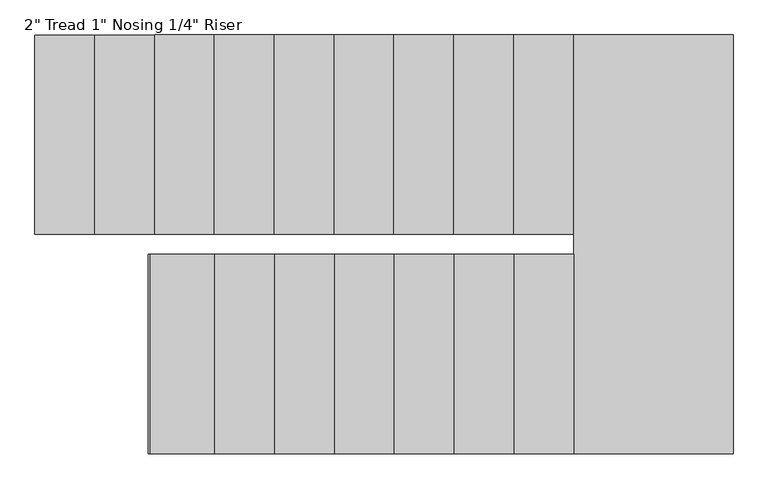
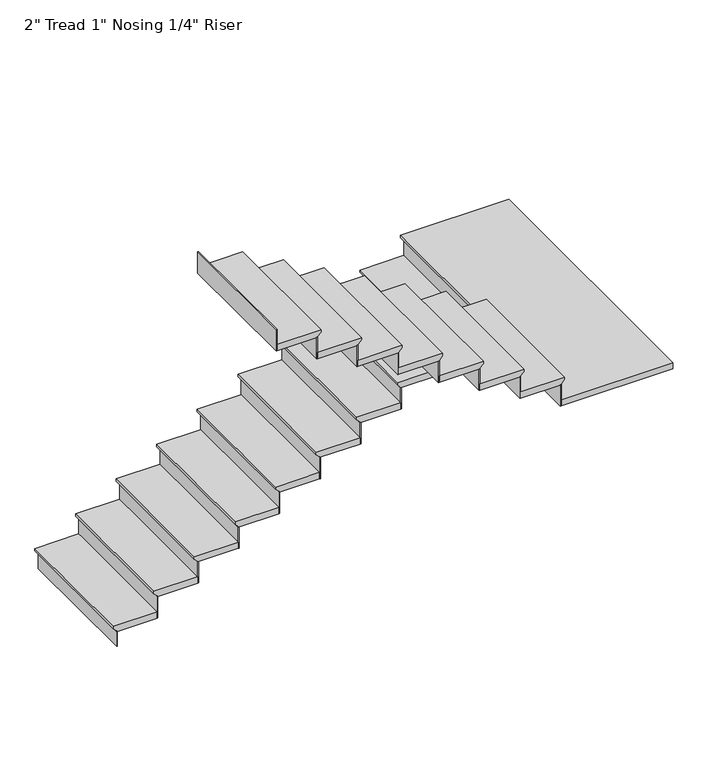
"""IFC4 building model written with IfcOpenShell, lengths in millimetres: stair flight geometry."""

from ifc_helpers import new_model, si_unit, origin, place, context, project, spatial, faceted_brep, source, transform, mapped, element, save


def stair_flight_7f10be43(model_context):
    return source(origin(), model_context, "Body", "Brep", [
        faceted_brep([(-12755.7436606, -2894.3024127, 3503.0833333), (-12755.7436606, -2894.3024127, 3522.1333333), (-12755.7436606, -1878.3024127, 3522.1333333), (-12755.7436606, -1878.3024127, 3503.0833333), (-12730.3436606, -2894.3024127, 3477.6833333), (-12730.3436606, -1878.3024127, 3477.6833333), (-12425.5436606, -2894.3024127, 3522.1333333), (-12425.5436606, -1878.3024127, 3522.1333333), (-12730.3436606, -1878.3024127, 3471.3333333), (-12425.5436606, -1878.3024127, 3471.3333333), (-12425.5436606, -2894.3024127, 3471.3333333), (-12730.3436606, -2894.3024127, 3471.3333333)], [[[0, 1, 2, 3]], [[4, 0, 3, 5]], [[2, 1, 6, 7]], [[8, 9, 10, 11]], [[2, 7, 9, 8, 5, 3]], [[8, 11, 4, 5]], [[6, 1, 0, 4, 11, 10]], [[7, 6, 10, 9]]]),
        faceted_brep([(-12730.3436606, -2894.3024127, 3471.3333333), (-12730.3436606, -2894.3024127, 3352.8), (-12723.9936606, -2894.3024127, 3352.8), (-12723.9936606, -2894.3024127, 3471.3333333), (-12730.3436606, -1878.3024127, 3471.3333333), (-12723.9936606, -1878.3024127, 3471.3333333), (-12723.9936606, -1878.3024127, 3352.8), (-12730.3436606, -1878.3024127, 3352.8)], [[[0, 1, 2, 3]], [[4, 5, 6, 7]], [[1, 0, 4, 7]], [[2, 1, 7, 6]], [[3, 2, 6, 5]], [[0, 3, 5, 4]]]),
        faceted_brep([(-12425.5436606, -2894.3024127, 3640.6666667), (-12425.5436606, -2894.3024127, 3471.3333333), (-12419.1936606, -2894.3024127, 3471.3333333), (-12419.1936606, -2894.3024127, 3640.6666667), (-12425.5436606, -1878.3024127, 3640.6666667), (-12419.1936606, -1878.3024127, 3640.6666667), (-12419.1936606, -1878.3024127, 3471.3333333), (-12425.5436606, -1878.3024127, 3471.3333333)], [[[0, 1, 2, 3]], [[4, 5, 6, 7]], [[1, 0, 4, 7]], [[2, 1, 7, 6]], [[3, 2, 6, 5]], [[0, 3, 5, 4]]]),
        faceted_brep([(-12450.9436606, -1878.3024127, 3691.4666667), (-12450.9436606, -2894.3024127, 3691.4666667), (-12120.7436606, -2894.3024127, 3691.4666667), (-12120.7436606, -1878.3024127, 3691.4666667), (-12425.5436606, -1878.3024127, 3640.6666667), (-12120.7436606, -1878.3024127, 3640.6666667), (-12120.7436606, -2894.3024127, 3640.6666667), (-12425.5436606, -2894.3024127, 3640.6666667), (-12425.5436606, -1878.3024127, 3647.0166667), (-12450.9436606, -1878.3024127, 3672.4166667), (-12425.5436606, -2894.3024127, 3647.0166667), (-12450.9436606, -2894.3024127, 3672.4166667)], [[[0, 1, 2, 3]], [[4, 5, 6, 7]], [[0, 3, 5, 4, 8, 9]], [[4, 7, 10, 8]], [[2, 1, 11, 10, 7, 6]], [[3, 2, 6, 5]], [[11, 1, 0, 9]], [[10, 11, 9, 8]]]),
        faceted_brep([(-12120.7436606, -2894.3024127, 3810.0), (-12120.7436606, -2894.3024127, 3640.6666667), (-12114.3936606, -2894.3024127, 3640.6666667), (-12114.3936606, -2894.3024127, 3810.0), (-12120.7436606, -1878.3024127, 3810.0), (-12114.3936606, -1878.3024127, 3810.0), (-12114.3936606, -1878.3024127, 3640.6666667), (-12120.7436606, -1878.3024127, 3640.6666667)], [[[0, 1, 2, 3]], [[4, 5, 6, 7]], [[1, 0, 4, 7]], [[2, 1, 7, 6]], [[3, 2, 6, 5]], [[0, 3, 5, 4]]]),
        faceted_brep([(-12146.1436606, -1878.3024127, 3860.8), (-12146.1436606, -2894.3024127, 3860.8), (-11815.9436606, -2894.3024127, 3860.8), (-11815.9436606, -1878.3024127, 3860.8), (-12120.7436606, -1878.3024127, 3810.0), (-11815.9436606, -1878.3024127, 3810.0), (-11815.9436606, -2894.3024127, 3810.0), (-12120.7436606, -2894.3024127, 3810.0), (-12120.7436606, -1878.3024127, 3816.35), (-12146.1436606, -1878.3024127, 3841.75), (-12120.7436606, -2894.3024127, 3816.35), (-12146.1436606, -2894.3024127, 3841.75)], [[[0, 1, 2, 3]], [[4, 5, 6, 7]], [[0, 3, 5, 4, 8, 9]], [[4, 7, 10, 8]], [[2, 1, 11, 10, 7, 6]], [[3, 2, 6, 5]], [[11, 1, 0, 9]], [[10, 11, 9, 8]]]),
        faceted_brep([(-11815.9436606, -2894.3024127, 3979.3333333), (-11815.9436606, -2894.3024127, 3810.0), (-11809.5936606, -2894.3024127, 3810.0), (-11809.5936606, -2894.3024127, 3979.3333333), (-11815.9436606, -1878.3024127, 3979.3333333), (-11809.5936606, -1878.3024127, 3979.3333333), (-11809.5936606, -1878.3024127, 3810.0), (-11815.9436606, -1878.3024127, 3810.0)], [[[0, 1, 2, 3]], [[4, 5, 6, 7]], [[1, 0, 4, 7]], [[2, 1, 7, 6]], [[3, 2, 6, 5]], [[0, 3, 5, 4]]]),
        faceted_brep([(-11841.3436606, -1878.3024127, 4030.1333333), (-11841.3436606, -2894.3024127, 4030.1333333), (-11511.1436606, -2894.3024127, 4030.1333333), (-11511.1436606, -1878.3024127, 4030.1333333), (-11815.9436606, -1878.3024127, 3979.3333333), (-11511.1436606, -1878.3024127, 3979.3333333), (-11511.1436606, -2894.3024127, 3979.3333333), (-11815.9436606, -2894.3024127, 3979.3333333), (-11815.9436606, -1878.3024127, 3985.6833333), (-11841.3436606, -1878.3024127, 4011.0833333), (-11815.9436606, -2894.3024127, 3985.6833333), (-11841.3436606, -2894.3024127, 4011.0833333)], [[[0, 1, 2, 3]], [[4, 5, 6, 7]], [[0, 3, 5, 4, 8, 9]], [[4, 7, 10, 8]], [[2, 1, 11, 10, 7, 6]], [[3, 2, 6, 5]], [[11, 1, 0, 9]], [[10, 11, 9, 8]]]),
        faceted_brep([(-11511.1436606, -2894.3024127, 4148.6666667), (-11511.1436606, -2894.3024127, 3979.3333333), (-11504.7936606, -2894.3024127, 3979.3333333), (-11504.7936606, -2894.3024127, 4148.6666667), (-11511.1436606, -1878.3024127, 4148.6666667), (-11504.7936606, -1878.3024127, 4148.6666667), (-11504.7936606, -1878.3024127, 3979.3333333), (-11511.1436606, -1878.3024127, 3979.3333333)], [[[0, 1, 2, 3]], [[4, 5, 6, 7]], [[1, 0, 4, 7]], [[2, 1, 7, 6]], [[3, 2, 6, 5]], [[0, 3, 5, 4]]]),
        faceted_brep([(-11536.5436606, -1878.3024127, 4199.4666667), (-11536.5436606, -2894.3024127, 4199.4666667), (-11206.3436606, -2894.3024127, 4199.4666667), (-11206.3436606, -1878.3024127, 4199.4666667), (-11511.1436606, -1878.3024127, 4148.6666667), (-11206.3436606, -1878.3024127, 4148.6666667), (-11206.3436606, -2894.3024127, 4148.6666667), (-11511.1436606, -2894.3024127, 4148.6666667), (-11511.1436606, -1878.3024127, 4155.0166667), (-11536.5436606, -1878.3024127, 4180.4166667), (-11511.1436606, -2894.3024127, 4155.0166667), (-11536.5436606, -2894.3024127, 4180.4166667)], [[[0, 1, 2, 3]], [[4, 5, 6, 7]], [[0, 3, 5, 4, 8, 9]], [[4, 7, 10, 8]], [[2, 1, 11, 10, 7, 6]], [[3, 2, 6, 5]], [[11, 1, 0, 9]], [[10, 11, 9, 8]]]),
        faceted_brep([(-11206.3436606, -2894.3024127, 4318.0), (-11206.3436606, -2894.3024127, 4148.6666667), (-11199.9936606, -2894.3024127, 4148.6666667), (-11199.9936606, -2894.3024127, 4318.0), (-11206.3436606, -1878.3024127, 4318.0), (-11199.9936606, -1878.3024127, 4318.0), (-11199.9936606, -1878.3024127, 4148.6666667), (-11206.3436606, -1878.3024127, 4148.6666667)], [[[0, 1, 2, 3]], [[4, 5, 6, 7]], [[1, 0, 4, 7]], [[2, 1, 7, 6]], [[3, 2, 6, 5]], [[0, 3, 5, 4]]]),
        faceted_brep([(-11231.7436606, -1878.3024127, 4368.8), (-11231.7436606, -2894.3024127, 4368.8), (-10901.5436606, -2894.3024127, 4368.8), (-10901.5436606, -1878.3024127, 4368.8), (-11206.3436606, -1878.3024127, 4318.0), (-10901.5436606, -1878.3024127, 4318.0), (-10901.5436606, -2894.3024127, 4318.0), (-11206.3436606, -2894.3024127, 4318.0), (-11206.3436606, -1878.3024127, 4324.35), (-11231.7436606, -1878.3024127, 4349.75), (-11206.3436606, -2894.3024127, 4324.35), (-11231.7436606, -2894.3024127, 4349.75)], [[[0, 1, 2, 3]], [[4, 5, 6, 7]], [[0, 3, 5, 4, 8, 9]], [[4, 7, 10, 8]], [[2, 1, 11, 10, 7, 6]], [[3, 2, 6, 5]], [[11, 1, 0, 9]], [[10, 11, 9, 8]]]),
        faceted_brep([(-10901.5436606, -2894.3024127, 4487.3333333), (-10901.5436606, -2894.3024127, 4318.0), (-10895.1936606, -2894.3024127, 4318.0), (-10895.1936606, -2894.3024127, 4487.3333333), (-10901.5436606, -1878.3024127, 4487.3333333), (-10895.1936606, -1878.3024127, 4487.3333333), (-10895.1936606, -1878.3024127, 4318.0), (-10901.5436606, -1878.3024127, 4318.0)], [[[0, 1, 2, 3]], [[4, 5, 6, 7]], [[1, 0, 4, 7]], [[2, 1, 7, 6]], [[3, 2, 6, 5]], [[0, 3, 5, 4]]]),
        faceted_brep([(-10926.9436606, -1878.3024127, 4538.1333333), (-10926.9436606, -2894.3024127, 4538.1333333), (-10596.7436606, -2894.3024127, 4538.1333333), (-10596.7436606, -1878.3024127, 4538.1333333), (-10901.5436606, -1878.3024127, 4487.3333333), (-10596.7436606, -1878.3024127, 4487.3333333), (-10596.7436606, -2894.3024127, 4487.3333333), (-10901.5436606, -2894.3024127, 4487.3333333), (-10901.5436606, -1878.3024127, 4493.6833333), (-10926.9436606, -1878.3024127, 4519.0833333), (-10901.5436606, -2894.3024127, 4493.6833333), (-10926.9436606, -2894.3024127, 4519.0833333)], [[[0, 1, 2, 3]], [[4, 5, 6, 7]], [[0, 3, 5, 4, 8, 9]], [[4, 7, 10, 8]], [[2, 1, 11, 10, 7, 6]], [[3, 2, 6, 5]], [[11, 1, 0, 9]], [[10, 11, 9, 8]]]),
        faceted_brep([(-10596.7436606, -2894.3024127, 4656.6666667), (-10596.7436606, -2894.3024127, 4487.3333333), (-10590.3936606, -2894.3024127, 4487.3333333), (-10590.3936606, -2894.3024127, 4656.6666667), (-10596.7436606, -1878.3024127, 4656.6666667), (-10590.3936606, -1878.3024127, 4656.6666667), (-10590.3936606, -1878.3024127, 4487.3333333), (-10596.7436606, -1878.3024127, 4487.3333333)], [[[0, 1, 2, 3]], [[4, 5, 6, 7]], [[1, 0, 4, 7]], [[2, 1, 7, 6]], [[3, 2, 6, 5]], [[0, 3, 5, 4]]]),
        faceted_brep([(-10622.1436606, -1878.3024127, 4707.4666667), (-10622.1436606, -2894.3024127, 4707.4666667), (-10291.9436606, -2894.3024127, 4707.4666667), (-10291.9436606, -1878.3024127, 4707.4666667), (-10596.7436606, -1878.3024127, 4656.6666667), (-10291.9436606, -1878.3024127, 4656.6666667), (-10291.9436606, -2894.3024127, 4656.6666667), (-10596.7436606, -2894.3024127, 4656.6666667), (-10596.7436606, -1878.3024127, 4663.0166667), (-10622.1436606, -1878.3024127, 4688.4166667), (-10596.7436606, -2894.3024127, 4663.0166667), (-10622.1436606, -2894.3024127, 4688.4166667)], [[[0, 1, 2, 3]], [[4, 5, 6, 7]], [[0, 3, 5, 4, 8, 9]], [[4, 7, 10, 8]], [[2, 1, 11, 10, 7, 6]], [[3, 2, 6, 5]], [[11, 1, 0, 9]], [[10, 11, 9, 8]]]),
        faceted_brep([(-10291.9436606, -2894.3024127, 4826.0), (-10291.9436606, -2894.3024127, 4656.6666667), (-10285.5936606, -2894.3024127, 4656.6666667), (-10285.5936606, -2894.3024127, 4826.0), (-10291.9436606, -1878.3024127, 4826.0), (-10285.5936606, -1878.3024127, 4826.0), (-10285.5936606, -1878.3024127, 4656.6666667), (-10291.9436606, -1878.3024127, 4656.6666667)], [[[0, 1, 2, 3]], [[4, 5, 6, 7]], [[1, 0, 4, 7]], [[2, 1, 7, 6]], [[3, 2, 6, 5]], [[0, 3, 5, 4]]]),
        faceted_brep([(-10317.3436606, -1878.3024127, 4876.8), (-10317.3436606, -2894.3024127, 4876.8), (-9987.1436606, -2894.3024127, 4876.8), (-9987.1436606, -1878.3024127, 4876.8), (-10291.9436606, -1878.3024127, 4826.0), (-9987.1436606, -1878.3024127, 4826.0), (-9987.1436606, -2894.3024127, 4826.0), (-10291.9436606, -2894.3024127, 4826.0), (-10291.9436606, -1878.3024127, 4832.35), (-10317.3436606, -1878.3024127, 4857.75), (-10291.9436606, -2894.3024127, 4832.35), (-10317.3436606, -2894.3024127, 4857.75)], [[[0, 1, 2, 3]], [[4, 5, 6, 7]], [[0, 3, 5, 4, 8, 9]], [[4, 7, 10, 8]], [[2, 1, 11, 10, 7, 6]], [[3, 2, 6, 5]], [[11, 1, 0, 9]], [[10, 11, 9, 8]]]),
        faceted_brep([(-9987.1436606, -2894.3024127, 4995.3333333), (-9987.1436606, -2894.3024127, 4826.0), (-9980.7936606, -2894.3024127, 4826.0), (-9980.7936606, -2894.3024127, 4995.3333333), (-9987.1436606, -1878.3024127, 4995.3333333), (-9980.7936606, -1878.3024127, 4995.3333333), (-9980.7936606, -1878.3024127, 4826.0), (-9987.1436606, -1878.3024127, 4826.0)], [[[0, 1, 2, 3]], [[4, 5, 6, 7]], [[1, 0, 4, 7]], [[2, 1, 7, 6]], [[3, 2, 6, 5]], [[0, 3, 5, 4]]]),
        faceted_brep([(-10037.9436606, -4011.9024127, 5046.1333333), (-9199.7436606, -4011.9024127, 5046.1333333), (-9199.7436606, -1878.3024127, 5046.1333333), (-10012.5436606, -1878.3024127, 5046.1333333), (-10012.5436606, -2995.9024127, 5046.1333333), (-10037.9436606, -2995.9024127, 5046.1333333), (-9199.7436606, -4011.9024127, 4995.3333333), (-10037.9436606, -4011.9024127, 4995.3333333), (-10037.9436606, -2995.9024127, 4995.3333333), (-10012.5436606, -2995.9024127, 4995.3333333), (-10012.5436606, -2894.3024127, 4995.3333333), (-9987.1436606, -2894.3024127, 4995.3333333), (-9987.1436606, -1878.3024127, 4995.3333333), (-9199.7436606, -1878.3024127, 4995.3333333), (-9987.1436606, -1878.3024127, 5001.6833333), (-10012.5436606, -1878.3024127, 5027.0833333), (-9987.1436606, -2894.3024127, 5001.6833333), (-10012.5436606, -2894.3024127, 5027.0833333)], [[[0, 1, 2, 3, 4, 5]], [[6, 7, 8, 9, 10, 11, 12, 13]], [[1, 0, 7, 6]], [[2, 1, 6, 13]], [[3, 2, 13, 12, 14, 15]], [[12, 11, 16, 14]], [[11, 10, 17, 16]], [[4, 3, 15, 17, 10, 9]], [[5, 4, 9, 8]], [[0, 5, 8, 7]], [[15, 14, 16, 17]]]),
        faceted_brep([(-10037.9436606, -2995.9024127, 5164.6666667), (-10037.9436606, -2995.9024127, 4995.3333333), (-10044.2936606, -2995.9024127, 4995.3333333), (-10044.2936606, -2995.9024127, 5164.6666667), (-10037.9436606, -4011.9024127, 5164.6666667), (-10044.2936606, -4011.9024127, 5164.6666667), (-10044.2936606, -4011.9024127, 4995.3333333), (-10037.9436606, -4011.9024127, 4995.3333333)], [[[0, 1, 2, 3]], [[4, 5, 6, 7]], [[1, 0, 4, 7]], [[2, 1, 7, 6]], [[3, 2, 6, 5]], [[0, 3, 5, 4]]]),
        faceted_brep([(-10012.5436606, -4011.9024127, 5215.4666667), (-10012.5436606, -2995.9024127, 5215.4666667), (-10342.7436606, -2995.9024127, 5215.4666667), (-10342.7436606, -4011.9024127, 5215.4666667), (-10037.9436606, -4011.9024127, 5164.6666667), (-10342.7436606, -4011.9024127, 5164.6666667), (-10342.7436606, -2995.9024127, 5164.6666667), (-10037.9436606, -2995.9024127, 5164.6666667), (-10037.9436606, -4011.9024127, 5171.0166667), (-10012.5436606, -4011.9024127, 5196.4166667), (-10037.9436606, -2995.9024127, 5171.0166667), (-10012.5436606, -2995.9024127, 5196.4166667)], [[[0, 1, 2, 3]], [[4, 5, 6, 7]], [[0, 3, 5, 4, 8, 9]], [[4, 7, 10, 8]], [[2, 1, 11, 10, 7, 6]], [[3, 2, 6, 5]], [[11, 1, 0, 9]], [[10, 11, 9, 8]]]),
        faceted_brep([(-10342.7436606, -2995.9024127, 5334.0), (-10342.7436606, -2995.9024127, 5164.6666667), (-10349.0936606, -2995.9024127, 5164.6666667), (-10349.0936606, -2995.9024127, 5334.0), (-10342.7436606, -4011.9024127, 5334.0), (-10349.0936606, -4011.9024127, 5334.0), (-10349.0936606, -4011.9024127, 5164.6666667), (-10342.7436606, -4011.9024127, 5164.6666667)], [[[0, 1, 2, 3]], [[4, 5, 6, 7]], [[1, 0, 4, 7]], [[2, 1, 7, 6]], [[3, 2, 6, 5]], [[0, 3, 5, 4]]]),
        faceted_brep([(-10317.3436606, -4011.9024127, 5384.8), (-10317.3436606, -2995.9024127, 5384.8), (-10647.5436606, -2995.9024127, 5384.8), (-10647.5436606, -4011.9024127, 5384.8), (-10342.7436606, -4011.9024127, 5334.0), (-10647.5436606, -4011.9024127, 5334.0), (-10647.5436606, -2995.9024127, 5334.0), (-10342.7436606, -2995.9024127, 5334.0), (-10342.7436606, -4011.9024127, 5340.35), (-10317.3436606, -4011.9024127, 5365.75), (-10342.7436606, -2995.9024127, 5340.35), (-10317.3436606, -2995.9024127, 5365.75)], [[[0, 1, 2, 3]], [[4, 5, 6, 7]], [[0, 3, 5, 4, 8, 9]], [[4, 7, 10, 8]], [[2, 1, 11, 10, 7, 6]], [[3, 2, 6, 5]], [[11, 1, 0, 9]], [[10, 11, 9, 8]]]),
        faceted_brep([(-10647.5436606, -2995.9024127, 5503.3333333), (-10647.5436606, -2995.9024127, 5334.0), (-10653.8936606, -2995.9024127, 5334.0), (-10653.8936606, -2995.9024127, 5503.3333333), (-10647.5436606, -4011.9024127, 5503.3333333), (-10653.8936606, -4011.9024127, 5503.3333333), (-10653.8936606, -4011.9024127, 5334.0), (-10647.5436606, -4011.9024127, 5334.0)], [[[0, 1, 2, 3]], [[4, 5, 6, 7]], [[1, 0, 4, 7]], [[2, 1, 7, 6]], [[3, 2, 6, 5]], [[0, 3, 5, 4]]]),
        faceted_brep([(-10622.1436606, -4011.9024127, 5554.1333333), (-10622.1436606, -2995.9024127, 5554.1333333), (-10952.3436606, -2995.9024127, 5554.1333333), (-10952.3436606, -4011.9024127, 5554.1333333), (-10647.5436606, -4011.9024127, 5503.3333333), (-10952.3436606, -4011.9024127, 5503.3333333), (-10952.3436606, -2995.9024127, 5503.3333333), (-10647.5436606, -2995.9024127, 5503.3333333), (-10647.5436606, -4011.9024127, 5509.6833333), (-10622.1436606, -4011.9024127, 5535.0833333), (-10647.5436606, -2995.9024127, 5509.6833333), (-10622.1436606, -2995.9024127, 5535.0833333)], [[[0, 1, 2, 3]], [[4, 5, 6, 7]], [[0, 3, 5, 4, 8, 9]], [[4, 7, 10, 8]], [[2, 1, 11, 10, 7, 6]], [[3, 2, 6, 5]], [[11, 1, 0, 9]], [[10, 11, 9, 8]]]),
        faceted_brep([(-10952.3436606, -2995.9024127, 5672.6666667), (-10952.3436606, -2995.9024127, 5503.3333333), (-10958.6936606, -2995.9024127, 5503.3333333), (-10958.6936606, -2995.9024127, 5672.6666667), (-10952.3436606, -4011.9024127, 5672.6666667), (-10958.6936606, -4011.9024127, 5672.6666667), (-10958.6936606, -4011.9024127, 5503.3333333), (-10952.3436606, -4011.9024127, 5503.3333333)], [[[0, 1, 2, 3]], [[4, 5, 6, 7]], [[1, 0, 4, 7]], [[2, 1, 7, 6]], [[3, 2, 6, 5]], [[0, 3, 5, 4]]]),
        faceted_brep([(-10926.9436606, -4011.9024127, 5723.4666667), (-10926.9436606, -2995.9024127, 5723.4666667), (-11257.1436606, -2995.9024127, 5723.4666667), (-11257.1436606, -4011.9024127, 5723.4666667), (-10952.3436606, -4011.9024127, 5672.6666667), (-11257.1436606, -4011.9024127, 5672.6666667), (-11257.1436606, -2995.9024127, 5672.6666667), (-10952.3436606, -2995.9024127, 5672.6666667), (-10952.3436606, -4011.9024127, 5679.0166667), (-10926.9436606, -4011.9024127, 5704.4166667), (-10952.3436606, -2995.9024127, 5679.0166667), (-10926.9436606, -2995.9024127, 5704.4166667)], [[[0, 1, 2, 3]], [[4, 5, 6, 7]], [[0, 3, 5, 4, 8, 9]], [[4, 7, 10, 8]], [[2, 1, 11, 10, 7, 6]], [[3, 2, 6, 5]], [[11, 1, 0, 9]], [[10, 11, 9, 8]]]),
        faceted_brep([(-11257.1436606, -2995.9024127, 5842.0), (-11257.1436606, -2995.9024127, 5672.6666667), (-11263.4936606, -2995.9024127, 5672.6666667), (-11263.4936606, -2995.9024127, 5842.0), (-11257.1436606, -4011.9024127, 5842.0), (-11263.4936606, -4011.9024127, 5842.0), (-11263.4936606, -4011.9024127, 5672.6666667), (-11257.1436606, -4011.9024127, 5672.6666667)], [[[0, 1, 2, 3]], [[4, 5, 6, 7]], [[1, 0, 4, 7]], [[2, 1, 7, 6]], [[3, 2, 6, 5]], [[0, 3, 5, 4]]]),
        faceted_brep([(-11231.7436606, -4011.9024127, 5892.8), (-11231.7436606, -2995.9024127, 5892.8), (-11561.9436606, -2995.9024127, 5892.8), (-11561.9436606, -4011.9024127, 5892.8), (-11257.1436606, -4011.9024127, 5842.0), (-11561.9436606, -4011.9024127, 5842.0), (-11561.9436606, -2995.9024127, 5842.0), (-11257.1436606, -2995.9024127, 5842.0), (-11257.1436606, -4011.9024127, 5848.35), (-11231.7436606, -4011.9024127, 5873.75), (-11257.1436606, -2995.9024127, 5848.35), (-11231.7436606, -2995.9024127, 5873.75)], [[[0, 1, 2, 3]], [[4, 5, 6, 7]], [[0, 3, 5, 4, 8, 9]], [[4, 7, 10, 8]], [[2, 1, 11, 10, 7, 6]], [[3, 2, 6, 5]], [[11, 1, 0, 9]], [[10, 11, 9, 8]]]),
        faceted_brep([(-11561.9436606, -2995.9024127, 6011.3333333), (-11561.9436606, -2995.9024127, 5842.0), (-11568.2936606, -2995.9024127, 5842.0), (-11568.2936606, -2995.9024127, 6011.3333333), (-11561.9436606, -4011.9024127, 6011.3333333), (-11568.2936606, -4011.9024127, 6011.3333333), (-11568.2936606, -4011.9024127, 5842.0), (-11561.9436606, -4011.9024127, 5842.0)], [[[0, 1, 2, 3]], [[4, 5, 6, 7]], [[1, 0, 4, 7]], [[2, 1, 7, 6]], [[3, 2, 6, 5]], [[0, 3, 5, 4]]]),
        faceted_brep([(-11536.5436606, -4011.9024127, 6062.1333333), (-11536.5436606, -2995.9024127, 6062.1333333), (-11866.7436606, -2995.9024127, 6062.1333333), (-11866.7436606, -4011.9024127, 6062.1333333), (-11561.9436606, -4011.9024127, 6011.3333333), (-11866.7436606, -4011.9024127, 6011.3333333), (-11866.7436606, -2995.9024127, 6011.3333333), (-11561.9436606, -2995.9024127, 6011.3333333), (-11561.9436606, -4011.9024127, 6017.6833333), (-11536.5436606, -4011.9024127, 6043.0833333), (-11561.9436606, -2995.9024127, 6017.6833333), (-11536.5436606, -2995.9024127, 6043.0833333)], [[[0, 1, 2, 3]], [[4, 5, 6, 7]], [[0, 3, 5, 4, 8, 9]], [[4, 7, 10, 8]], [[2, 1, 11, 10, 7, 6]], [[3, 2, 6, 5]], [[11, 1, 0, 9]], [[10, 11, 9, 8]]]),
        faceted_brep([(-11866.7436606, -2995.9024127, 6180.6666667), (-11866.7436606, -2995.9024127, 6011.3333333), (-11873.0936606, -2995.9024127, 6011.3333333), (-11873.0936606, -2995.9024127, 6180.6666667), (-11866.7436606, -4011.9024127, 6180.6666667), (-11873.0936606, -4011.9024127, 6180.6666667), (-11873.0936606, -4011.9024127, 6011.3333333), (-11866.7436606, -4011.9024127, 6011.3333333)], [[[0, 1, 2, 3]], [[4, 5, 6, 7]], [[1, 0, 4, 7]], [[2, 1, 7, 6]], [[3, 2, 6, 5]], [[0, 3, 5, 4]]]),
        faceted_brep([(-12171.5436606, -2995.9024127, 6350.0), (-12171.5436606, -2995.9024127, 6180.6666667), (-12177.8936606, -2995.9024127, 6180.6666667), (-12177.8936606, -2995.9024127, 6350.0), (-12171.5436606, -4011.9024127, 6350.0), (-12177.8936606, -4011.9024127, 6350.0), (-12177.8936606, -4011.9024127, 6180.6666667), (-12171.5436606, -4011.9024127, 6180.6666667)], [[[0, 1, 2, 3]], [[4, 5, 6, 7]], [[1, 0, 4, 7]], [[2, 1, 7, 6]], [[3, 2, 6, 5]], [[0, 3, 5, 4]]]),
        faceted_brep([(-11841.3436606, -4011.9024127, 6231.4666667), (-11841.3436606, -2995.9024127, 6231.4666667), (-12171.5436606, -2995.9024127, 6231.4666667), (-12171.5436606, -4011.9024127, 6231.4666667), (-11866.7436606, -4011.9024127, 6180.6666667), (-12171.5436606, -4011.9024127, 6180.6666667), (-12171.5436606, -2995.9024127, 6180.6666667), (-11866.7436606, -2995.9024127, 6180.6666667), (-11866.7436606, -4011.9024127, 6187.0166667), (-11841.3436606, -4011.9024127, 6212.4166667), (-11866.7436606, -2995.9024127, 6187.0166667), (-11841.3436606, -2995.9024127, 6212.4166667)], [[[0, 1, 2, 3]], [[4, 5, 6, 7]], [[0, 3, 5, 4, 8, 9]], [[4, 7, 10, 8]], [[2, 1, 11, 10, 7, 6]], [[3, 2, 6, 5]], [[11, 1, 0, 9]], [[10, 11, 9, 8]]]),
    ])


if __name__ == "__main__":
    model = new_model("IFC4")
    model_context = context("Model", 3, world=origin())
    ifc_project = project(units=[si_unit("LENGTHUNIT", "METRE", prefix="MILLI")], contexts=[model_context])
    site = spatial("IfcSite", under=ifc_project)
    building = spatial("IfcBuilding", under=site)
    placement = place(None, origin())
    stair_flight_shape = stair_flight_7f10be43(model_context)
    element("IfcStairFlight", 1, ObjectType="2\" Tread 1\" Nosing 1/4\" Riser", at=placement, inside=building, context=model_context, shape_type="MappedRepresentation", body=[
        mapped(stair_flight_shape, transform((0.0, 0.0, 0.0), x_axis=(1.0, 0.0, 0.0), y_axis=(0.0, 1.0, 0.0), z_axis=(0.0, 0.0, 1.0))),
    ])
    save(model, "model.ifc")

# Revit data of these elements
# Element 1 (IfcStairFlight, "2\" Tread 1\" Nosing 1/4\" Riser")
#   Materials on its faces: "Clad - White"
# Materials
#   "Clad - White": class "Wood", colour RGB 30 30 30, transparency 0, Cost = 0
